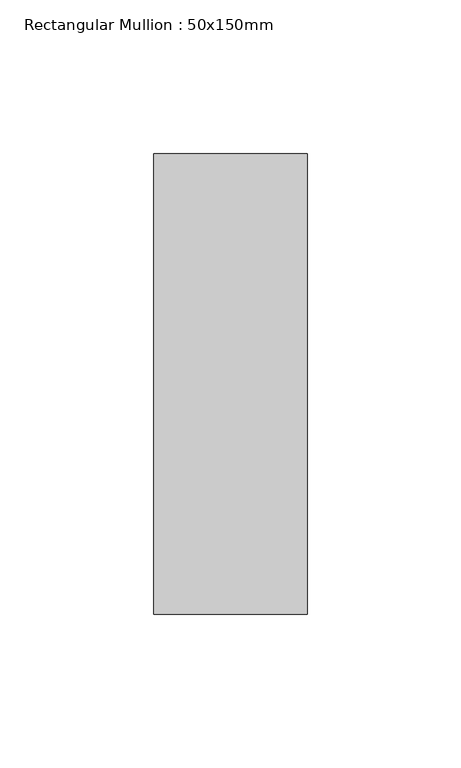
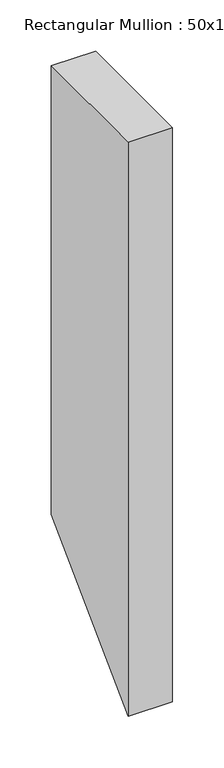
"""IFC4 building model written with IfcOpenShell, lengths in millimetres: member geometry, Rectangular Mullion : 50x150mm."""

from ifc_helpers import new_model, si_unit, frame, origin, place, context, project, spatial, polyline, outline, extrude, source, transform, mapped, element, save


def rectangular_mullion_50x150mm_d3e7ce4f(model_context):
    return source(origin(), model_context, "Body", "SweptSolid", [
        extrude(outline(polyline([(-75.0, 0.0), (75.0, 0.0), (75.0, -534.6), (-75.0, -684.6), (-75.0, 0.0)])), frame((-50.0, 0.0, 0.0), z_axis=(1.0, 0.0, 0.0), x_axis=(0.0, 1.0, 0.0)), (0.0, 0.0, 1.0), 50.0),
    ])


if __name__ == "__main__":
    model = new_model("IFC4")
    model_context = context("Model", 3, world=origin())
    ifc_project = project(units=[si_unit("LENGTHUNIT", "METRE", prefix="MILLI")], contexts=[model_context])
    site = spatial("IfcSite", under=ifc_project)
    building = spatial("IfcBuilding", under=site)
    placement = place(None, origin())
    rectangular_mullion_50x150mm_shape = rectangular_mullion_50x150mm_d3e7ce4f(model_context)
    element("IfcMember", 1, ObjectType="Rectangular Mullion : 50x150mm", at=placement, inside=building, context=model_context, shape_type="MappedRepresentation", body=[
        mapped(rectangular_mullion_50x150mm_shape, transform((0.0, 0.0, 0.0), x_axis=(1.0, 0.0, 0.0), y_axis=(0.0, 1.0, 0.0), z_axis=(0.0, 0.0, 1.0))),
    ])
    save(model, "model.ifc")

# Revit data of these elements
# Type "Rectangular Mullion : 50x150mm"
#   Keynote = "H11"
#   built-in parameter 1007304 = 0.492126 (stored number, unit not read)
#   built-in parameter 1007301 = 0.082021 (stored number, unit not read)
#   built-in parameter 1007300 = 0.082021 (stored number, unit not read)
# Element 1 (IfcMember, "Rectangular Mullion : 50x150mm")
#   Materials on its faces: "Aluminium"
# Materials
#   "Aluminium": class "Metal", colour RGB 247 247 247, transparency 0, Description = "Aluminium 6061", Cost = 0
